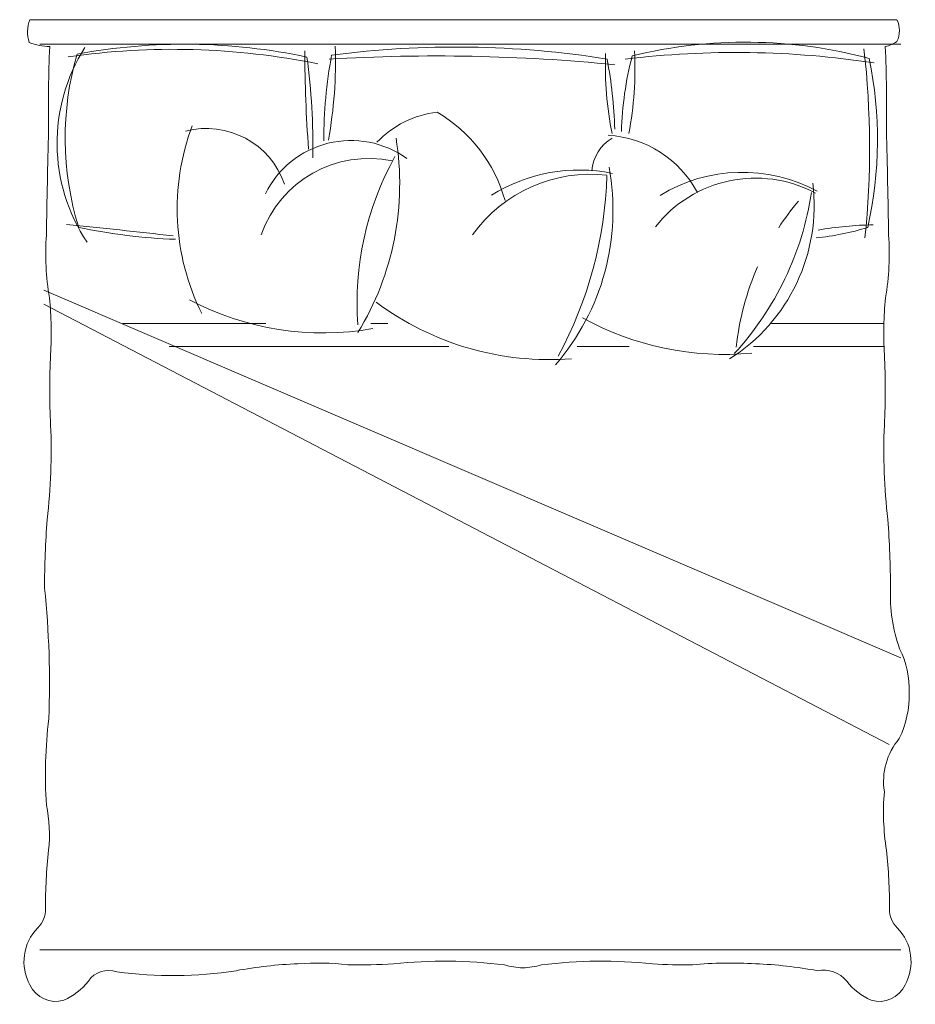
# Model space of a CAD drawing. Units: inches. Extents: x 2129 to 3258, y 1851 to 3021.
# Tile 9 of 10: x 3257.61643 to 3257.69344, y 2150.92167 to 2151.00629. Entities that reach past the tile are written whole.
import ezdxf

# ---------------------------------------------------------------- set-up
doc = ezdxf.new("R2010")
doc.units = ezdxf.units.IN
doc.layers.add('A-FURN', color=8, linetype='Continuous', lineweight=18)

# ---------------------------------------------------------------- blocks, each defined once
blk = doc.blocks.new('bed 1- king size')
at = {"color": 0}
for p, q in [((-0.9487, -0.0777), (0.9323, -0.0777)), ((-0.9394, -0.6151), (0.9323, -1.4177)), ((-0.9394, -0.6451), (0.9066, -1.6065)), ((-0.7682, -0.6873), (-0.4547, -0.6873)), ((-0.2254, -0.6873), (-0.1884, -0.6873)), ((0.6495, -0.6873), (0.8951, -0.6873)), ((-0.6659, -0.7381), (-0.0555, -0.7381)), ((0.2254, -0.7381), (0.3384, -0.7381)), ((0.6103, -0.7381), (0.8953, -0.7381)), ((-0.9487, -2.0547), (0.9323, -2.0547))]:
    blk.add_line(p, q, dxfattribs=at)
blk.add_lwpolyline([(0.898, -0.0829, 0.098699), (0.9236, -0.072, 0.222522), (0.9236, -0.0243), (-0.9705, -0.0243, 0.171621), (-0.9716, -0.0739, 0.102495), (-0.9268, -0.0829, 0.015571), (-0.9293, -0.2659, 0.00267), (-0.9341, -0.4944, 0.058958), (-0.9274, -0.6315, -0.038458), (-0.9248, -0.7552, 0.025508), (-0.9248, -0.9094, -0.039412), (-0.9326, -1.1154, 0.016498), (-0.9382, -1.2654, -0.035771), (-0.9288, -1.5502, 0.045388), (-0.9341, -1.7389, -0.080578), (-0.9295, -1.837, 0.026504), (-0.9362, -1.9656, -0.211134), (-0.9531, -2.0066, 0.329446), (-0.9701, -2.1314, 0.37589), (-0.8958, -2.1647, 0.123892), (-0.8425, -2.1233, -0.342539), (-0.78, -2.1029, 0.07104), (-0.5197, -2.1004, -0.036442), (-0.3847, -2.0853, -0.046791), (-0.2759, -2.0873, 0.023628), (-0.1759, -2.0852, -0.055897), (0.0662, -2.0877, 0.053528), (0.1067, -2.0945, 0.053528), (0.1472, -2.0877, -0.055897), (0.3893, -2.0852, 0.026973), (0.4769, -2.0873, -0.036947), (0.6147, -2.0853, -0.036442), (0.7497, -2.1004, -0.281256), (0.8137, -2.1233, -0.521995), (0.8137, -2.1233, 0.123892), (0.867, -2.1647, 0.37589), (0.9413, -2.1314, 0.329446), (0.9243, -2.0066, -0.211134), (0.9074, -1.9656, 0.026504), (0.9007, -1.837, -0.06219), (0.896, -1.7098, -0.218233), (0.9286, -1.5937, 0.123513), (0.9499, -1.4937, 0.129887), (0.9293, -1.3978, -0.095063), (0.9094, -1.2654, 0.016498), (0.9038, -1.1154, -0.039412), (0.896, -0.9094, 0.025508), (0.896, -0.7552, -0.038458), (0.8986, -0.6315, 0.058958), (0.9053, -0.4944, 0.00267), (0.9005, -0.2659, 0.015571)], format="xyb", close=True, dxfattribs=at)
for centre, radius, start, end in [((-0.5221, -0.2938), 0.3887, 147.51, 213.8336), ((-0.6323, -1.3651), 1.2872, 78.0142, 100.5125), ((-1.2482, -0.1161), 0.9455, 349.589, 2.0447), ((-0.04, -2.1818), 2.0978, 80.934, 97.4266), ((0.5931, -1.1167), 1.0433, 75.0181, 103.7392), ((-0.2311, -0.2827), 0.6619, 163.9263, 197.1409), ((-0.6569, -1.6774), 1.5884, 78.5485, 98.3029), ((2.5431, -0.0869), 2.9129, 180.1063, 184.3312), ((-1.857, -0.3037), 1.5051, 359.1536, 7.5533), ((0.7071, -0.2897), 1.0355, 169.5301, 179.934), ((-0.0818, -4.0689), 3.9654, 84.3658, 93.3969), ((1.0242, -0.1263), 0.7375, 177.8261, 191.4767), ((1.0572, -0.2894), 0.7358, 165.3434, 178.3876), ((0.5721, -2.1074), 2.0115, 81.3714, 96.917), ((-0.3946, -0.1329), 0.7459, 349.1667, 3.123), ((-1.0492, -0.3038), 1.9129, 354.0935, 6.4707), ((-0.6896, -0.2953), 0.9974, 1.8337, 10.6945), ((0.0089, -0.2863), 0.8722, 347.3175, 11.7435), ((-0.0546, -0.4435), 0.2189, 96.8992, 136.0421), ((-0.2438, -0.5051), 0.323, 15.4018, 59.7122), ((-0.1358, -0.4371), 0.5128, 159.3026, 206.5026), ((-0.5846, -0.4421), 0.1803, 18.9387, 104.6725), ((0.2786, -0.5137), 0.2374, 28.1996, 86.5061), ((-0.2688, -0.4962), 0.2082, 54.1671, 153.8421), ((-0.7873, -0.3825), 0.6248, 328.6542, 9.1977), ((0.347, -0.3604), 0.0899, 120.1134, 175.8974), ((-0.2301, -0.5756), 0.2484, 78.0413, 160.8342), ((0.4039, -0.6426), 0.6595, 151.0456, 184.1497), ((0.2545, -0.6795), 0.3178, 83.5607, 144.2853), ((0.2294, -0.7137), 0.3612, 78.4081, 122.0077), ((-0.2123, -0.4404), 0.5157, 319.1339, 10.5299), ((-0.5982, -0.336), 0.8889, 331.605, 358.1749), ((0.5856, -0.7025), 0.345, 61.6404, 121.3345), ((0.6148, -0.6485), 0.2783, 61.8876, 141.8707), ((0.3458, -0.4294), 0.3969, 302.3262, 7), ((0.0793, -0.3025), 0.6649, 317.3201, 351.4624), ((1.163, -0.8025), 0.5939, 139.9508, 146.951), ((-1.8444, -10.4721), 10.046, 83.21322, 84.54762), ((0.8799, -1.1936), 0.7214, 90.6432, 100.2707), ((-0.6059, 0.7469), 1.2515, 258.1169, 267.8849), ((0.6944, 0.0492), 0.5523, 275.447, 287.4199), ((1.163, -0.8025), 0.5939, 156.2982, 173.8539), ((-0.3293, -0.0779), 0.6301, 242.3859, 279.8951), ((0.1632, -0.137), 0.6293, 233.2201, 274.4972), ((0.5459, -0.118), 0.637, 240.9467, 275.467)]:
    blk.add_arc(centre, radius, start, end, dxfattribs=at)

msp = doc.modelspace()

# ---------------------------------------------------------------- block references
at = {"layer": 'A-FURN', "xscale": 0.0393700787401575, "yscale": 0.0393700787401575, "zscale": 0.0393700787401575}
msp.add_blockref('bed 1- king size', (3257.655507, 2151.007249), dxfattribs=at)

doc.saveas('drawing.dxf')
